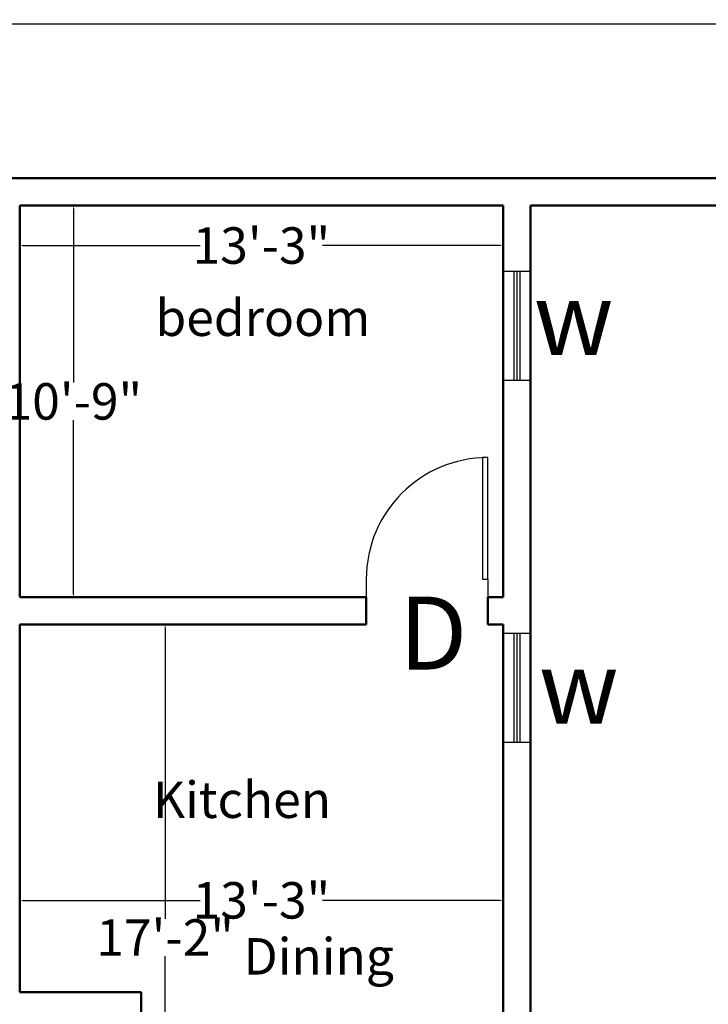
# Model space of a CAD drawing. Units: inches. Extents: x 409 to 7572, y 7 to 725.
# Tile 37 of 38: x 6994 to 7221, y 401 to 725. Entities that reach past the tile are written whole.
import ezdxf

# ---------------------------------------------------------------- set-up
doc = ezdxf.new("R2010")
doc.units = ezdxf.units.IN
doc.header["$MEASUREMENT"] = 0
for name, color, linetype, lineweight in [('A-ANNO-DIMS', 2, 'Continuous', 18), ('A-ANNO-SYMB', 3, 'Continuous', 25), ('A-AREA-IDEN', 7, 'Continuous', 25), ('A-DOOR', 3, 'Continuous', 25), ('A-GLAZ', 4, 'Continuous', 25), ('A-WALL', 7, 'Continuous', 50)]:
    doc.layers.add(name, color=color, linetype=linetype, lineweight=lineweight)
doc.styles.get("Standard").update_dxf_attribs({"font": 'arial.ttf'})
doc.dimstyles.get("Standard").update_dxf_attribs({"dimtxt": 2, "dimasz": 1, "dimexe": 0.18, "dimexo": 0.0625, "dimgap": 0.09, "dimtad": 0, "dimtih": 1, "dimtoh": 1, "dimdec": 0, "dimzin": 0, "dimdsep": 46, "dimlunit": 3, "dimtxsty": 'Standard', "dimcen": 0.09, "dimadec": 0, "dimazin": 0, "dimtfac": 1, "dimtdec": 0, "dimtofl": 0, "dimtmove": 0, "dimatfit": 3, "dimfxl": 1, "dimtolj": 1, "dimtzin": 0, "dimarcsym": 0})

# ---------------------------------------------------------------- blocks, each defined once
blk = doc.blocks.new('*U2')
for p, q in [((0, 0), (0, -6)), ((-40, 0), (-40, -6))]:
    blk.add_line(p, q)
blk.add_lwpolyline([(0, 0), (0, 40), (-1.75, 40), (-1.75, 0)], close=True)
blk.add_arc((0, 0), 40, 90, 180)
blk = doc.blocks.new('*D152')
at = {"layer": 'A-ANNO-DIMS', "color": 0, "lineweight": -2, "transparency": 16777216}
for p, q in [((6994.47, 663.53), (7012.24, 663.53)), ((7012.06, 662.53), (7012.06, 605.25)), ((7012.06, 535.53), (7012.06, 592.81)), ((6994.47, 534.53), (7012.24, 534.53))]:
    blk.add_line(p, q, dxfattribs=at)
at = {"layer": 'A-ANNO-DIMS', "color": 0, "transparency": 16777216}
for points in [[(7011.9, 662.53), (7012.23, 662.53), (7012.06, 663.53)], [(7011.9, 535.53), (7012.23, 535.53), (7012.06, 534.53)]]:
    blk.add_solid(points, dxfattribs=at)
at = {"layer": 'DEFPOINTS', "color": 0, "transparency": 16777216}
for p in [(6994.41, 663.53), (6994.41, 534.53), (7012.06, 534.53)]:
    blk.add_point(p, dxfattribs=at)
at = {"layer": 'A-ANNO-DIMS', "color": 0, "transparency": 16777216, "insert": (7012.06, 599.03), "char_height": 2, "attachment_point": 5}
blk.add_mtext('\\A1;{\\H6x;10\'-9"}', dxfattribs=at)
blk = doc.blocks.new('*D153')
at = {"layer": 'A-ANNO-DIMS', "color": 0, "lineweight": -2, "transparency": 16777216}
for p, q in [((6994.41, 663.47), (6994.41, 650.17)), ((7153.41, 663.47), (7153.41, 650.17)), ((6995.41, 650.35), (7053.78, 650.35)), ((7152.41, 650.35), (7094.05, 650.35))]:
    blk.add_line(p, q, dxfattribs=at)
at = {"layer": 'A-ANNO-DIMS', "color": 0, "transparency": 16777216}
for points in [[(6995.41, 650.52), (6995.41, 650.19), (6994.41, 650.35)], [(7152.41, 650.52), (7152.41, 650.19), (7153.41, 650.35)]]:
    blk.add_solid(points, dxfattribs=at)
at = {"layer": 'DEFPOINTS', "color": 0, "transparency": 16777216}
for p in [(6994.41, 663.53), (7153.41, 663.53), (7153.41, 650.35)]:
    blk.add_point(p, dxfattribs=at)
at = {"layer": 'A-ANNO-DIMS', "color": 0, "transparency": 16777216, "insert": (7073.91, 650.35), "char_height": 2, "attachment_point": 5}
blk.add_mtext('\\A1;{\\H6x;13\'-3"}', dxfattribs=at)
blk = doc.blocks.new('*D157')
at = {"layer": 'A-ANNO-DIMS', "color": 0, "lineweight": -2, "transparency": 16777216}
for p, q in [((6994.41, 404.59), (6994.41, 434.95)), ((6995.41, 434.77), (7053.78, 434.77)), ((7152.41, 434.77), (7094.05, 434.77)), ((7153.41, 404.59), (7153.41, 434.95))]:
    blk.add_line(p, q, dxfattribs=at)
at = {"layer": 'A-ANNO-DIMS', "color": 0, "transparency": 16777216}
for points in [[(6995.41, 434.93), (6995.41, 434.6), (6994.41, 434.77)], [(7152.41, 434.93), (7152.41, 434.6), (7153.41, 434.77)]]:
    blk.add_solid(points, dxfattribs=at)
at = {"layer": 'DEFPOINTS', "color": 0, "transparency": 16777216}
for p in [(7153.41, 434.77), (6994.41, 404.53), (7153.41, 404.53)]:
    blk.add_point(p, dxfattribs=at)
at = {"layer": 'A-ANNO-DIMS', "color": 0, "transparency": 16777216, "insert": (7073.91, 434.77), "char_height": 2, "attachment_point": 5}
blk.add_mtext('\\A1;{\\H6x;13\'-3"}', dxfattribs=at)
blk = doc.blocks.new('*D158')
at = {"layer": 'A-ANNO-DIMS', "color": 0, "lineweight": -2, "transparency": 16777216}
for p, q in [((7051.35, 525.53), (7042.07, 525.53)), ((7042.25, 524.53), (7042.25, 428.65)), ((7042.25, 320.53), (7042.25, 416.42)), ((7059.35, 319.53), (7042.07, 319.53))]:
    blk.add_line(p, q, dxfattribs=at)
at = {"layer": 'A-ANNO-DIMS', "color": 0, "transparency": 16777216}
for points in [[(7042.08, 524.53), (7042.42, 524.53), (7042.25, 525.53)], [(7042.08, 320.53), (7042.42, 320.53), (7042.25, 319.53)]]:
    blk.add_solid(points, dxfattribs=at)
at = {"layer": 'DEFPOINTS', "color": 0, "transparency": 16777216}
for p in [(7051.41, 525.53), (7042.25, 319.53), (7059.41, 319.53)]:
    blk.add_point(p, dxfattribs=at)
at = {"layer": 'A-ANNO-DIMS', "color": 0, "transparency": 16777216, "insert": (7042.25, 422.53), "char_height": 2, "attachment_point": 5}
blk.add_mtext('\\A1;{\\H6x;17\'-2"}', dxfattribs=at)
blk = doc.blocks.new('*D161')
at = {"layer": 'A-ANNO-DIMS', "color": 0, "lineweight": -2, "transparency": 16777216}
for p, q in [((6985.41, 672.59), (6985.41, 723.56)), ((6986.41, 723.38), (7252.85, 723.38)), ((7526.41, 723.38), (7259.98, 723.38)), ((7527.41, 672.59), (7527.41, 723.56))]:
    blk.add_line(p, q, dxfattribs=at)
at = {"layer": 'A-ANNO-DIMS', "color": 0, "transparency": 16777216}
for points in [[(6986.41, 723.55), (6986.41, 723.22), (6985.41, 723.38)], [(7526.41, 723.55), (7526.41, 723.22), (7527.41, 723.38)]]:
    blk.add_solid(points, dxfattribs=at)
at = {"layer": 'DEFPOINTS', "color": 0, "transparency": 16777216}
for p in [(6985.41, 723.38), (6985.41, 672.53), (7527.41, 672.53)]:
    blk.add_point(p, dxfattribs=at)
at = {"layer": 'A-ANNO-DIMS', "color": 0, "transparency": 16777216, "insert": (7256.41, 723.38), "char_height": 2, "attachment_point": 5}
blk.add_mtext('\\A1;45\'-2"', dxfattribs=at)
blk = doc.blocks.new('WIN-36')
for p, q in [((1699.82, 514.65), (1699.82, 478.65)), ((1700.82, 514.65), (1700.82, 478.65)), ((1701.82, 514.65), (1701.82, 478.65))]:
    blk.add_line(p, q)
blk.add_lwpolyline([(1705.32, 514.65), (1705.32, 478.65), (1696.32, 478.65), (1696.32, 514.65)], close=True)

msp = doc.modelspace()

# ---------------------------------------------------------------- linework, layer by layer
at = {"layer": 'A-WALL'}
for p, q in [((7527.41, 672.53), (6985.41, 672.53)), ((7153.41, 663.53), (6994.41, 663.53)), ((6994.41, 663.53), (6994.41, 534.53)), ((7153.41, 663.53), (7153.41, 534.53)), ((7153.41, 663.53), (7153.41, 534.53)), ((7518.41, 663.53), (7162.41, 663.53)), ((7162.41, 663.53), (7162.41, 603.53)), ((7162.41, 663.53), (7162.41, 474.53)), ((7162.41, 663.53), (7162.41, 337.53)), ((7108.41, 534.53), (6994.41, 534.53)), ((7108.41, 534.53), (7108.41, 525.53)), ((7153.41, 534.53), (7148.41, 534.53)), ((7148.41, 534.53), (7148.41, 525.53)), ((7108.41, 525.53), (6994.41, 525.53)), ((6994.41, 525.53), (6994.41, 404.53)), ((7153.41, 525.53), (7148.41, 525.53)), ((7153.41, 525.53), (7153.41, 319.53)), ((7034.41, 404.53), (6994.41, 404.53)), ((7034.41, 404.53), (7034.41, 395.53))]:
    msp.add_line(p, q, dxfattribs=at)

# ---------------------------------------------------------------- block references
at = {"layer": 'A-DOOR'}
msp.add_blockref('*U2', (7148.41, 540.53), dxfattribs=at)
at = {"layer": 'A-GLAZ'}
for p in [(5457.09, 127.23), (5457.09, 8.1)]:
    msp.add_blockref('WIN-36', p, dxfattribs=at)

# ---------------------------------------------------------------- texts
at = {"layer": 'A-ANNO-SYMB', "char_height": 24, "attachment_point": 1}
for s, width, insert in [('w', 18.2582, (7163.49, 638.33)), ('D', 19.1972, (7119.13, 534.75)), ('w', 18.2582, (7165.18, 516.97))]:
    msp.add_mtext_dynamic_manual_height_columns(s, width=width, gutter_width=1, heights=[0], dxfattribs=dict(at, insert=insert))
at = {"layer": 'A-AREA-IDEN', "char_height": 12, "attachment_point": 1}
for s, width, insert in [('bedroom', 40.9017, (7039.07, 632.57)), ('Kitchen ', 61.5504, (7038.24, 473.89)), ('Dining ', 67.5069, (7068.02, 422.33))]:
    msp.add_mtext_dynamic_manual_height_columns(s, width=width, gutter_width=1, heights=[0], dxfattribs=dict(at, insert=insert))

# ---------------------------------------------------------------- dimensions: what is measured, and where the dimension line sits
at = {"layer": 'A-ANNO-DIMS'}
dim = msp.add_linear_dim(base=(6985.41, 723.38), p1=(7527.41, 672.53), p2=(6985.41, 672.53), dimstyle='Standard', override={"dimclrd": 0, "dimclre": 0, "dimclrt": 0}, dxfattribs=at)
dim.commit()
dim.dimension.update_dxf_attribs({"geometry": '*D161', "text_midpoint": (7256.41, 723.38)})
dim = msp.add_linear_dim(base=(7012.06, 534.53), p1=(6994.41, 663.53), p2=(6994.41, 534.53), angle=90, text='{\\H6x;<>}', dimstyle='Standard', override={"dimclrd": 0, "dimclre": 0, "dimclrt": 0}, dxfattribs=at)
dim.commit()
dim.dimension.update_dxf_attribs({"geometry": '*D152', "text_midpoint": (7012.06, 599.03)})
for base, p1, p2, picture, middle in [((7153.41, 650.35), (6994.41, 663.53), (7153.41, 663.53), '*D153', (7073.91, 650.35)), ((7153.41, 434.77), (6994.41, 404.53), (7153.41, 404.53), '*D157', (7073.91, 434.77))]:
    dim = msp.add_linear_dim(base=base, p1=p1, p2=p2, text='{\\H6x;<>}', dimstyle='Standard', override={"dimclrd": 0, "dimclre": 0, "dimclrt": 0}, dxfattribs=at)
    dim.commit()
    dim.dimension.update_dxf_attribs({"geometry": picture, "text_midpoint": middle})
dim = msp.add_linear_dim(base=(7042.25, 319.53), p1=(7051.41, 525.53), p2=(7059.41, 319.53), angle=90, text='{\\H6x;<>}', dimstyle='Standard', override={"dimclrd": 0, "dimclre": 0, "dimclrt": 0}, dxfattribs=at)
dim.commit()
dim.dimension.update_dxf_attribs({"geometry": '*D158', "text_midpoint": (7042.25, 422.53), "dimtype": 160})

doc.saveas('drawing.dxf')
